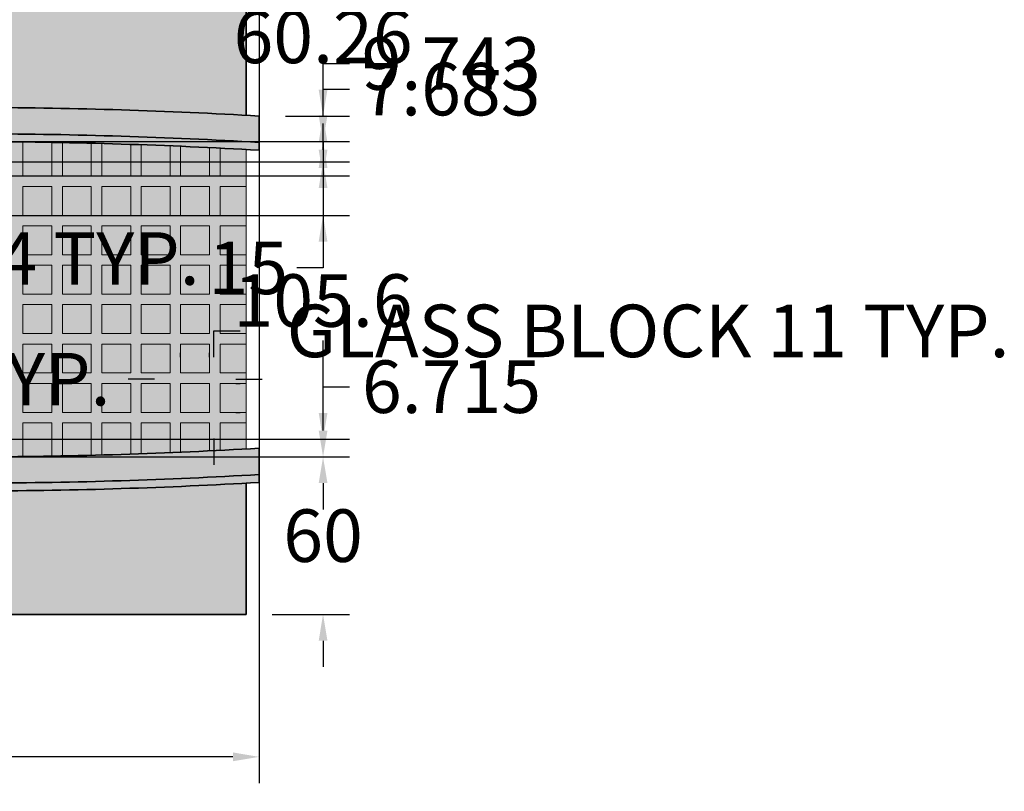
# Model space of a CAD drawing. Units: millimetres. Extents: x 130 to 1021, y 147 to 699.
# Tile 39 of 40: x 646 to 1021, y 147 to 440. Entities that reach past the tile are written whole.
import ezdxf

# ---------------------------------------------------------------- set-up
doc = ezdxf.new("R2010")
doc.units = ezdxf.units.MM
doc.header["$MEASUREMENT"] = 0
for name, color, linetype, lineweight in [('A-ANNO-DIMS', 2, 'Continuous', 18), ('A-ELEV', 7, 'Continuous', 35), ('A-ELEV-PATT', 9, 'Continuous', 13), ('A-GLAZ', 4, 'Continuous', 18)]:
    doc.layers.add(name, color=color, linetype=linetype, lineweight=lineweight)
doc.styles.get("Standard").update_dxf_attribs({"font": 'arial.ttf'})
doc.dimstyles.get("Standard").update_dxf_attribs({"dimtxt": 20, "dimasz": 10, "dimexe": 10, "dimexo": 10, "dimgap": 5, "dimtad": 0, "dimtih": 1, "dimtoh": 1, "dimdec": 0, "dimzin": 0, "dimdsep": 46, "dimtxsty": 'Standard', "dimcen": 5, "dimadec": 0, "dimazin": 0, "dimtfac": 1, "dimtdec": 0, "dimtofl": 0, "dimtmove": 0, "dimatfit": 3, "dimfxl": 1, "dimtolj": 1, "dimtzin": 0, "dimarcsym": 0})

# ---------------------------------------------------------------- blocks, each defined once
blk = doc.blocks.new('GLASS-BLOCK')
for p, q in [((0, 0), (0, 11)), ((0, 11), (11, 11)), ((11, 0), (11, 11)), ((0, 0), (11, 0))]:
    blk.add_line(p, q)
blk = doc.blocks.new('*D5')
at = {"layer": 'A-ANNO-DIMS', "color": 0, "lineweight": -2, "transparency": 16777216}
for p, q in [((720.13, 311.89), (720.13, 321.89)), ((720.13, 321.89), (730.13, 321.89)), ((728.48, 301.89), (730.13, 301.89)), ((728.48, 290.89), (730.13, 290.89)), ((720.13, 280.89), (720.13, 270.89))]:
    blk.add_line(p, q, dxfattribs=at)
at = {"layer": 'A-ANNO-DIMS', "color": 0, "transparency": 16777216}
for points in [[(718.46, 311.89), (721.8, 311.89), (720.13, 301.89)], [(718.46, 280.89), (721.8, 280.89), (720.13, 290.89)]]:
    blk.add_solid(points, dxfattribs=at)
at = {"layer": 'Defpoints', "color": 0, "transparency": 16777216}
for p in [(718.48, 301.89), (720.13, 301.89), (718.48, 290.89)]:
    blk.add_point(p, dxfattribs=at)
at = {"layer": 'A-ANNO-DIMS', "color": 0, "transparency": 16777216, "insert": (885.35, 321.89), "char_height": 20, "attachment_point": 5}
blk.add_mtext('\\A1;GLASS BLOCK 11 TYP.', dxfattribs=at)
blk = doc.blocks.new('*D6')
at = {"layer": 'A-ANNO-DIMS', "color": 0, "lineweight": -2, "transparency": 16777216}
for p, q in [((707.48, 311.89), (707.48, 313.54)), ((718.48, 311.89), (718.48, 313.54)), ((697.48, 303.54), (687.48, 303.54)), ((728.48, 303.54), (738.48, 303.54))]:
    blk.add_line(p, q, dxfattribs=at)
at = {"layer": 'A-ANNO-DIMS', "color": 0, "transparency": 16777216}
for points in [[(697.48, 305.21), (697.48, 301.87), (707.48, 303.54)], [(728.48, 305.21), (728.48, 301.87), (718.48, 303.54)]]:
    blk.add_solid(points, dxfattribs=at)
at = {"layer": 'Defpoints', "color": 0, "transparency": 16777216}
for p in [(707.48, 303.54), (707.48, 301.89), (718.48, 301.89)]:
    blk.add_point(p, dxfattribs=at)
at = {"layer": 'A-ANNO-DIMS', "color": 0, "transparency": 16777216, "insert": (634.74, 303.54), "char_height": 20, "attachment_point": 5}
blk.add_mtext('\\A1;11 TYP.', dxfattribs=at)
blk = doc.blocks.new('*D7')
at = {"layer": 'A-ANNO-DIMS', "color": 0, "lineweight": -2, "transparency": 16777216}
for p, q in [((399.37, 349.45), (413.37, 349.45)), ((423.37, 349.45), (433.37, 349.45)), ((389.37, 344.55), (389.37, 339.45)), ((423.37, 344.55), (423.37, 339.45))]:
    blk.add_line(p, q, dxfattribs=at)
at = {"layer": 'A-ANNO-DIMS', "color": 0, "transparency": 16777216}
for points in [[(399.37, 351.11), (399.37, 347.78), (389.37, 349.45)], [(413.37, 351.11), (413.37, 347.78), (423.37, 349.45)]]:
    blk.add_solid(points, dxfattribs=at)
at = {"layer": 'Defpoints', "color": 0, "transparency": 16777216}
for p in [(389.37, 354.55), (423.37, 354.55), (423.37, 349.45)]:
    blk.add_point(p, dxfattribs=at)
at = {"layer": 'A-ANNO-DIMS', "color": 0, "transparency": 16777216, "insert": (582.04, 349.45), "char_height": 20, "attachment_point": 5}
blk.add_mtext('\\A1;DOOR PANEL 34 TYP.', dxfattribs=at)
blk = doc.blocks.new('*D11')
at = {"layer": 'A-ANNO-DIMS', "color": 0, "lineweight": -2, "transparency": 16777216}
for p, q in [((737.37, 648.7), (737.37, 149.74)), ((299.37, 566.95), (299.37, 149.74)), ((309.37, 159.74), (490.86, 159.74)), ((727.37, 159.74), (545.89, 159.74))]:
    blk.add_line(p, q, dxfattribs=at)
at = {"layer": 'A-ANNO-DIMS', "color": 0, "transparency": 16777216}
for points in [[(309.37, 161.41), (309.37, 158.07), (299.37, 159.74)], [(727.37, 161.41), (727.37, 158.07), (737.37, 159.74)]]:
    blk.add_solid(points, dxfattribs=at)
at = {"layer": 'Defpoints', "color": 0, "transparency": 16777216}
for p in [(737.37, 658.7), (299.37, 576.95), (737.37, 159.74)]:
    blk.add_point(p, dxfattribs=at)
at = {"layer": 'A-ANNO-DIMS', "color": 0, "transparency": 16777216, "insert": (518.37, 159.74), "char_height": 20, "attachment_point": 5}
blk.add_mtext('\\A1;438', dxfattribs=at)
blk = doc.blocks.new('*D49')
at = {"layer": 'A-ANNO-DIMS', "color": 0, "lineweight": -2, "transparency": 16777216}
for p, q in [((761.67, 283.95), (761.67, 293.95)), ((642.82, 273.95), (771.67, 273.95)), ((742.37, 213.95), (771.67, 213.95)), ((761.67, 203.95), (761.67, 193.95))]:
    blk.add_line(p, q, dxfattribs=at)
at = {"layer": 'A-ANNO-DIMS', "color": 0, "transparency": 16777216}
for points in [[(760.01, 283.95), (763.34, 283.95), (761.67, 273.95)], [(760.01, 203.95), (763.34, 203.95), (761.67, 213.95)]]:
    blk.add_solid(points, dxfattribs=at)
at = {"layer": 'Defpoints', "color": 0, "transparency": 16777216}
for p in [(632.82, 273.95), (761.67, 273.95), (732.37, 213.95)]:
    blk.add_point(p, dxfattribs=at)
at = {"layer": 'A-ANNO-DIMS', "color": 0, "transparency": 16777216, "insert": (761.67, 243.95), "char_height": 20, "attachment_point": 5}
blk.add_mtext('\\A1;60', dxfattribs=at)
blk = doc.blocks.new('*D50')
at = {"layer": 'A-ANNO-DIMS', "color": 0, "lineweight": -2, "transparency": 16777216}
for p, q in [((761.67, 290.66), (761.67, 300.66)), ((761.67, 300.66), (771.67, 300.66)), ((554.64, 280.66), (771.67, 280.66)), ((642.82, 273.95), (771.67, 273.95)), ((761.67, 263.95), (761.67, 253.95))]:
    blk.add_line(p, q, dxfattribs=at)
at = {"layer": 'A-ANNO-DIMS', "color": 0, "transparency": 16777216}
for points in [[(760.01, 290.66), (763.34, 290.66), (761.67, 280.66)], [(760.01, 263.95), (763.34, 263.95), (761.67, 273.95)]]:
    blk.add_solid(points, dxfattribs=at)
at = {"layer": 'Defpoints', "color": 0, "transparency": 16777216}
for p in [(544.64, 280.66), (761.67, 280.66), (632.82, 273.95)]:
    blk.add_point(p, dxfattribs=at)
at = {"layer": 'A-ANNO-DIMS', "color": 0, "transparency": 16777216, "insert": (810.55, 300.66), "char_height": 20, "attachment_point": 5}
blk.add_mtext('\\A1;6.715', dxfattribs=at)
blk = doc.blocks.new('*D51')
at = {"layer": 'A-ANNO-DIMS', "color": 0, "lineweight": -2, "transparency": 16777216}
for p, q in [((554.64, 386.26), (771.67, 386.26)), ((761.67, 376.26), (761.67, 348.67)), ((761.67, 290.66), (761.67, 318.25)), ((554.64, 280.66), (771.67, 280.66))]:
    blk.add_line(p, q, dxfattribs=at)
at = {"layer": 'A-ANNO-DIMS', "color": 0, "transparency": 16777216}
for points in [[(760.01, 376.26), (763.34, 376.26), (761.67, 386.26)], [(760.01, 290.66), (763.34, 290.66), (761.67, 280.66)]]:
    blk.add_solid(points, dxfattribs=at)
at = {"layer": 'Defpoints', "color": 0, "transparency": 16777216}
for p in [(544.64, 386.26), (761.67, 386.26), (544.64, 280.66)]:
    blk.add_point(p, dxfattribs=at)
at = {"layer": 'A-ANNO-DIMS', "color": 0, "transparency": 16777216, "insert": (761.67, 333.46), "char_height": 20, "attachment_point": 5}
blk.add_mtext('\\A1;105.6', dxfattribs=at)
blk = doc.blocks.new('*D52')
at = {"layer": 'A-ANNO-DIMS', "color": 0, "lineweight": -2, "transparency": 16777216}
for p, q in [((761.67, 403.95), (761.67, 413.95)), ((761.67, 413.95), (771.67, 413.95)), ((642.82, 393.95), (771.67, 393.95)), ((554.64, 386.26), (771.67, 386.26)), ((761.67, 376.26), (761.67, 366.26))]:
    blk.add_line(p, q, dxfattribs=at)
at = {"layer": 'A-ANNO-DIMS', "color": 0, "transparency": 16777216}
for points in [[(760.01, 403.95), (763.34, 403.95), (761.67, 393.95)], [(760.01, 376.26), (763.34, 376.26), (761.67, 386.26)]]:
    blk.add_solid(points, dxfattribs=at)
at = {"layer": 'Defpoints', "color": 0, "transparency": 16777216}
for p in [(632.82, 393.95), (761.67, 393.95), (544.64, 386.26)]:
    blk.add_point(p, dxfattribs=at)
at = {"layer": 'A-ANNO-DIMS', "color": 0, "transparency": 16777216, "insert": (810.34, 413.95), "char_height": 20, "attachment_point": 5}
blk.add_mtext('\\A1;7.683', dxfattribs=at)
blk = doc.blocks.new('*D53')
at = {"layer": 'A-ANNO-DIMS', "color": 0, "lineweight": -2, "transparency": 16777216}
for p, q in [((761.67, 413.69), (761.67, 423.69)), ((761.67, 423.69), (771.67, 423.69)), ((747.37, 403.69), (771.67, 403.69)), ((642.82, 393.95), (771.67, 393.95)), ((761.67, 383.95), (761.67, 373.95))]:
    blk.add_line(p, q, dxfattribs=at)
at = {"layer": 'A-ANNO-DIMS', "color": 0, "transparency": 16777216}
for points in [[(760.01, 413.69), (763.34, 413.69), (761.67, 403.69)], [(760.01, 383.95), (763.34, 383.95), (761.67, 393.95)]]:
    blk.add_solid(points, dxfattribs=at)
at = {"layer": 'Defpoints', "color": 0, "transparency": 16777216}
for p in [(737.37, 403.69), (761.67, 403.69), (632.82, 393.95)]:
    blk.add_point(p, dxfattribs=at)
at = {"layer": 'A-ANNO-DIMS', "color": 0, "transparency": 16777216, "insert": (810.42, 423.69), "char_height": 20, "attachment_point": 5}
blk.add_mtext('\\A1;9.743', dxfattribs=at)
blk = doc.blocks.new('*D54')
at = {"layer": 'A-ANNO-DIMS', "color": 0, "lineweight": -2, "transparency": 16777216}
for p, q in [((761.67, 473.95), (761.67, 483.95)), ((497.37, 463.95), (771.67, 463.95)), ((747.37, 403.69), (771.67, 403.69)), ((761.67, 393.69), (761.67, 383.69))]:
    blk.add_line(p, q, dxfattribs=at)
at = {"layer": 'A-ANNO-DIMS', "color": 0, "transparency": 16777216}
for points in [[(760.01, 473.95), (763.34, 473.95), (761.67, 463.95)], [(760.01, 393.69), (763.34, 393.69), (761.67, 403.69)]]:
    blk.add_solid(points, dxfattribs=at)
at = {"layer": 'Defpoints', "color": 0, "transparency": 16777216}
for p in [(487.37, 463.95), (761.67, 463.95), (737.37, 403.69)]:
    blk.add_point(p, dxfattribs=at)
at = {"layer": 'A-ANNO-DIMS', "color": 0, "transparency": 16777216, "insert": (761.67, 433.82), "char_height": 20, "attachment_point": 5}
blk.add_mtext('\\A1;60.26', dxfattribs=at)
blk = doc.blocks.new('*D61')
at = {"layer": 'A-ANNO-DIMS', "color": 0, "lineweight": -2, "transparency": 16777216}
for p, q in [((761.67, 390.89), (761.67, 400.89)), ((642.82, 380.89), (771.67, 380.89)), ((642.82, 365.89), (771.67, 365.89)), ((761.67, 355.89), (761.67, 345.89)), ((761.67, 345.89), (751.67, 345.89))]:
    blk.add_line(p, q, dxfattribs=at)
at = {"layer": 'A-ANNO-DIMS', "color": 0, "transparency": 16777216}
for points in [[(760.01, 390.89), (763.34, 390.89), (761.67, 380.89)], [(760.01, 355.89), (763.34, 355.89), (761.67, 365.89)]]:
    blk.add_solid(points, dxfattribs=at)
at = {"layer": 'Defpoints', "color": 0, "transparency": 16777216}
for p in [(632.82, 380.89), (632.82, 365.89), (761.67, 365.89)]:
    blk.add_point(p, dxfattribs=at)
at = {"layer": 'A-ANNO-DIMS', "color": 0, "transparency": 16777216, "insert": (733.22, 345.89), "char_height": 20, "attachment_point": 5}
blk.add_mtext('\\A1;15', dxfattribs=at)

msp = doc.modelspace()

# ---------------------------------------------------------------- hatches: boundary and pattern name
at = {"layer": 'A-ELEV-PATT'}
h = msp.add_hatch(color=256, dxfattribs=at)
h.dxf.hatch_style = 1
h.paths.add_polyline_path([(737.3738, 658.6988, 0.01359606), (632.4019, 661.9473), (607.3738, 661.9473), (487.3738, 661.9473), (487.3738, 649.9473), (607.3738, 649.9473), (632.3794, 649.9473, -0.01368411), (737.3738, 646.6784)])
h.paths.add_polyline_path([(732.3738, 643.9599, 0.01305286), (632.3738, 646.9473), (607.3738, 646.9473), (487.3738, 646.9473), (487.3738, 596.9473), (632.3738, 596.9473, -0.01305286), (732.3738, 593.9599)])
h.paths.add_polyline_path([(737.3738, 593.6732, 0.01370629), (632.3738, 596.9473), (487.3738, 596.9473), (487.3738, 586.9473), (632.355, 586.9473, -0.01378075), (737.3738, 583.6559)])
h.paths.add_polyline_path([(447.3738, 646.9473), (307.3738, 646.9473), (302.3738, 646.9473), (302.3738, 634.9473), (447.3738, 634.9473)])
h.paths.add_polyline_path([(447.3738, 631.9473), (307.3738, 631.9473), (307.3738, 586.9473), (447.3738, 586.9473)])
h.paths.add_polyline_path([(447.3738, 586.9473), (307.3738, 586.9473), (302.3738, 586.9473), (302.3738, 576.9473), (447.3738, 576.9473)])
h.paths.add_polyline_path([(447.3738, 573.9473), (367.3738, 573.9473), (367.3738, 539.9473), (447.3738, 539.9473)])
h.paths.add_polyline_path([(447.3738, 537.9473), (367.3738, 537.9473), (367.3738, 507.9473), (400.392, 507.4253, -0.00172798), (401.3281, 507.6451, -0.52200255), (425.6117, 511.0391, -0.03918489), (447.3738, 510.4359), (447.3738, 510.7883)])
h.paths.add_polyline_path([(394.7238, 505.9473), (367.3738, 505.9473), (367.3738, 476.9473, -0.0146512), (375.8501, 480.2159), (376.1506, 499.2266, -0.03554194)])
h.paths.add_polyline_path([(632.3738, 583.9473), (552.3738, 583.9473), (552.3738, 550.9473), (632.3738, 550.9473)])
h.paths.add_polyline_path([(632.3738, 548.9473), (552.3738, 548.9473), (552.3738, 515.9473), (632.3738, 515.9473)])
h.paths.add_polyline_path([(632.3738, 513.9473), (552.3738, 513.9473), (552.3738, 476.9473), (632.3738, 476.9473)])
h.paths.add_polyline_path([(737.3738, 473.6903, 0.01363261), (632.3926, 476.9473), (552.3738, 476.9473), (487.3738, 476.9473), (487.3738, 466.9473), (632.3738, 466.9473, -0.01370629), (737.3738, 463.6732)])
h.paths.add_polyline_path([(732.3738, 460.9552, 0.01307409), (632.3681, 463.9473), (487.3738, 463.9473), (487.3738, 407.735, -0.00322862), (489.3544, 406.9473), (632.3926, 406.9473, -0.01298259), (732.3738, 403.9755)])
h.paths.add_polyline_path([(487.3738, 463.9473, 0.20132998), (367.3738, 463.9473), (367.3738, 407.735, -0.18820307), (487.3738, 407.735)])
h.paths.add_polyline_path([(367.3738, 476.9473), (367.3738, 466.9473, -0.20133085), (487.3738, 466.9473), (487.3738, 476.9473, 0.20132998)])
h.paths.add_polyline_path([(367.3738, 463.9473), (307.3738, 463.9473), (307.3738, 401.9473), (357.9413, 401.9473), (367.3738, 407.735)])
h.paths.add_polyline_path([(367.3738, 476.9473), (302.3738, 476.9473), (302.3738, 466.9473), (367.3738, 466.9473)])
h.paths.add_polyline_path([(632.8184, 366.9453), (552.3738, 366.9453), (552.3738, 393.9473), (632.8184, 393.9473)])
h.paths.add_polyline_path([(632.8184, 357.2114), (632.8184, 363.9453), (552.3738, 363.9453), (552.3738, 357.2114), (552.3738, 336.9453), (632.8184, 336.9453)])
h.paths.add_polyline_path([(632.8184, 333.9453), (552.3738, 333.9453), (552.3738, 306.9453), (632.8184, 306.9453)])
h.paths.add_polyline_path([(632.8184, 303.9453), (552.3738, 303.9453), (552.3738, 273.9473), (632.355, 273.9473, 0.00006077), (632.8184, 273.9491)])
h.paths.add_polyline_path([(737.3738, 403.6903, 0.01363261), (632.3926, 406.9473), (489.3544, 406.9473, 0.19154808), (367.3738, 407.735), (367.3738, 396.9473, -0.20133085), (487.3738, 396.9473), (632.3738, 396.9473, -0.01370629), (737.3738, 393.6732)])
h.paths.add_polyline_path([(357.9413, 401.9473), (307.3738, 401.9473), (307.3738, 391.9473), (357.9413, 391.9473)])
h.paths.add_polyline_path([(357.9413, 357.2114), (357.9413, 388.9473), (307.3738, 388.9473), (307.3738, 357.2114), (307.3738, 273.9473), (357.9413, 273.9473)])
h.paths.add_polyline_path([(732.3738, 263.93, -0.0130317), (632.3794, 260.9473), (466.7667, 260.9473), (466.7667, 240.9473), (469.8406, 236.978), (469.8406, 221.978), (472.9145, 218.0087), (472.9145, 213.9473), (607.3738, 213.9473), (732.3738, 213.9473)])
h.paths.add_polyline_path([(732.3738, 290.889), (722.479, 290.889), (722.479, 301.889), (732.3738, 301.889), (732.3738, 305.889), (722.479, 305.889), (722.479, 316.889), (732.3738, 316.889), (732.3738, 320.889), (722.479, 320.889), (722.479, 331.889), (732.3738, 331.889), (732.3738, 335.889), (722.479, 335.889), (722.479, 346.889), (732.3738, 346.889), (732.3738, 350.889), (722.479, 350.889), (722.479, 361.889), (732.3738, 361.889), (732.3738, 365.889), (722.479, 365.889), (722.479, 376.889), (732.3738, 376.889), (732.3738, 380.889), (722.479, 380.889), (722.479, 391.4848, 0.00052326), (718.479, 391.6843), (718.479, 380.889), (707.479, 380.889), (707.479, 392.1896, 0.00052307), (703.479, 392.3576), (703.479, 380.889), (692.479, 380.889), (692.479, 392.7765, 0.00052292), (688.479, 392.9131), (688.479, 380.889), (677.479, 380.889), (677.479, 393.2456, 0.00052279), (673.479, 393.3508), (673.479, 380.889), (662.479, 380.889), (662.479, 393.597, 0.0005227), (658.479, 393.6709), (658.479, 380.889), (647.479, 380.889), (647.479, 393.8308, 0.00052264), (643.479, 393.8732), (643.479, 380.889), (632.8184, 380.889), (632.8184, 376.889), (643.479, 376.889), (643.479, 365.889), (632.8184, 365.889), (632.8184, 361.889), (643.479, 361.889), (643.479, 350.889), (632.8184, 350.889), (632.8184, 346.889), (643.479, 346.889), (643.479, 335.889), (632.8184, 335.889), (632.8184, 331.889), (643.479, 331.889), (643.479, 320.889), (632.8184, 320.889), (632.8184, 316.889), (643.479, 316.889), (643.479, 305.889), (632.8184, 305.889), (632.8184, 301.889), (643.479, 301.889), (643.479, 290.889), (632.8184, 290.889), (632.8184, 286.889), (643.479, 286.889), (643.479, 274.0217, 0.00052456), (647.479, 274.0643), (647.479, 286.889), (658.479, 286.889), (658.479, 274.2248, 0.00052462), (662.479, 274.2989), (662.479, 286.889), (673.479, 286.889), (673.479, 274.546, 0.00052471), (677.479, 274.6516), (677.479, 286.889), (688.479, 286.889), (688.479, 274.9853, 0.00052484), (692.479, 275.1224), (692.479, 286.889), (703.479, 286.889), (703.479, 275.5429, 0.000525), (707.479, 275.7115), (707.479, 286.889), (718.479, 286.889), (718.479, 276.2187, 0.00052519), (722.479, 276.4189), (722.479, 286.889), (732.3738, 286.889)])
h.paths.add_polyline_path([(718.479, 290.889), (707.479, 290.889), (707.479, 301.889), (718.479, 301.889)], flags=16)
h.paths.add_polyline_path([(703.479, 290.889), (692.479, 290.889), (692.479, 301.889), (703.479, 301.889)], flags=16)
h.paths.add_polyline_path([(718.479, 305.889), (707.479, 305.889), (707.479, 316.889), (718.479, 316.889)], flags=16)
h.paths.add_polyline_path([(703.479, 305.889), (692.479, 305.889), (692.479, 316.889), (703.479, 316.889)], flags=16)
h.paths.add_polyline_path([(688.479, 290.889), (677.479, 290.889), (677.479, 301.889), (688.479, 301.889)], flags=16)
h.paths.add_polyline_path([(718.479, 320.889), (707.479, 320.889), (707.479, 331.889), (718.479, 331.889)], flags=16)
h.paths.add_polyline_path([(688.479, 305.889), (677.479, 305.889), (677.479, 316.889), (688.479, 316.889)], flags=16)
h.paths.add_polyline_path([(703.479, 320.889), (692.479, 320.889), (692.479, 331.889), (703.479, 331.889)], flags=16)
h.paths.add_polyline_path([(688.479, 320.889), (677.479, 320.889), (677.479, 331.889), (688.479, 331.889)], flags=16)
h.paths.add_polyline_path([(673.479, 290.889), (662.479, 290.889), (662.479, 301.889), (673.479, 301.889)], flags=16)
h.paths.add_polyline_path([(718.479, 335.889), (707.479, 335.889), (707.479, 346.889), (718.479, 346.889)], flags=16)
h.paths.add_polyline_path([(673.479, 305.889), (662.479, 305.889), (662.479, 316.889), (673.479, 316.889)], flags=16)
h.paths.add_polyline_path([(703.479, 335.889), (692.479, 335.889), (692.479, 346.889), (703.479, 346.889)], flags=16)
h.paths.add_polyline_path([(673.479, 320.889), (662.479, 320.889), (662.479, 331.889), (673.479, 331.889)], flags=16)
h.paths.add_polyline_path([(688.479, 335.889), (677.479, 335.889), (677.479, 346.889), (688.479, 346.889)], flags=16)
h.paths.add_polyline_path([(658.479, 290.889), (647.479, 290.889), (647.479, 301.889), (658.479, 301.889)], flags=16)
h.paths.add_polyline_path([(718.479, 350.889), (707.479, 350.889), (707.479, 361.889), (718.479, 361.889)], flags=16)
h.paths.add_polyline_path([(658.479, 305.889), (647.479, 305.889), (647.479, 316.889), (658.479, 316.889)], flags=16)
h.paths.add_polyline_path([(703.479, 350.889), (692.479, 350.889), (692.479, 361.889), (703.479, 361.889)], flags=16)
h.paths.add_polyline_path([(673.479, 335.889), (662.479, 335.889), (662.479, 346.889), (673.479, 346.889)], flags=16)
h.paths.add_polyline_path([(658.479, 320.889), (647.479, 320.889), (647.479, 331.889), (658.479, 331.889)], flags=16)
h.paths.add_polyline_path([(688.479, 350.889), (677.479, 350.889), (677.479, 361.889), (688.479, 361.889)], flags=16)
h.paths.add_polyline_path([(718.479, 365.889), (707.479, 365.889), (707.479, 376.889), (718.479, 376.889)], flags=16)
h.paths.add_polyline_path([(658.479, 335.889), (647.479, 335.889), (647.479, 346.889), (658.479, 346.889)], flags=16)
h.paths.add_polyline_path([(673.479, 350.889), (662.479, 350.889), (662.479, 361.889), (673.479, 361.889)], flags=16)
h.paths.add_polyline_path([(703.479, 365.889), (692.479, 365.889), (692.479, 376.889), (703.479, 376.889)], flags=16)
h.paths.add_polyline_path([(688.479, 365.889), (677.479, 365.889), (677.479, 376.889), (688.479, 376.889)], flags=16)
h.paths.add_polyline_path([(658.479, 350.889), (647.479, 350.889), (647.479, 361.889), (658.479, 361.889)], flags=16)
h.paths.add_polyline_path([(673.479, 365.889), (662.479, 365.889), (662.479, 376.889), (673.479, 376.889)], flags=16)
h.paths.add_polyline_path([(658.479, 365.889), (647.479, 365.889), (647.479, 376.889), (658.479, 376.889)], flags=16)
h.paths.add_polyline_path([(732.3738, 503.9786), (722.3392, 503.9786), (722.3392, 514.9786), (732.3738, 514.9786), (732.3738, 518.9786), (722.3392, 518.9786), (722.3392, 529.9786), (732.3738, 529.9786), (732.3738, 533.9786), (722.3392, 533.9786), (722.3392, 544.9786), (732.3738, 544.9786), (732.3738, 546.9473), (732.3738, 548.9786), (722.3392, 548.9786), (722.3392, 559.9786), (732.3738, 559.9786), (732.3738, 563.9786), (722.3392, 563.9786), (722.3392, 574.9786), (732.3738, 574.9786), (732.3738, 578.9786), (722.3392, 578.9786), (722.3392, 581.4789, 0.00052601), (718.3392, 581.6791), (718.3392, 578.9786), (707.3392, 578.9786), (707.3392, 582.1863, 0.00052582), (703.3392, 582.355), (703.3392, 578.9786), (692.3392, 578.9786), (692.3392, 582.7752, 0.00052566), (688.3392, 582.9123), (688.3392, 578.9786), (677.3392, 578.9786), (677.3392, 583.2457, 0.00052554), (673.3392, 583.3512), (673.3392, 578.9786), (662.3392, 578.9786), (662.3392, 583.5978, 0.00052545), (658.3392, 583.6718), (658.3392, 578.9786), (647.3392, 578.9786), (647.3392, 583.8317, 0.00052539), (643.3392, 583.8741), (643.3392, 578.9786), (632.3738, 578.9786), (632.3738, 574.9786), (643.3392, 574.9786), (643.3392, 563.9786), (632.3738, 563.9786), (632.3738, 559.9786), (643.3392, 559.9786), (643.3392, 548.9786), (632.3738, 548.9786), (632.3738, 544.9786), (643.3392, 544.9786), (643.3392, 533.9786), (632.3738, 533.9786), (632.3738, 529.9786), (643.3392, 529.9786), (643.3392, 518.9786), (632.3738, 518.9786), (632.3738, 515.9473), (632.3738, 514.9786), (643.3392, 514.9786), (643.3392, 503.9786), (632.3738, 503.9786), (632.3738, 499.9786), (643.3392, 499.9786), (643.3392, 488.9786), (632.3738, 488.9786), (632.3738, 484.9786), (643.3392, 484.9786), (643.3392, 476.8751, -0.00051911), (647.3392, 476.8332), (647.3392, 484.9786), (658.3392, 484.9786), (658.3392, 476.6752, -0.00051917), (662.3392, 476.6022), (662.3392, 484.9786), (673.3392, 484.9786), (673.3392, 476.3585, -0.00051926), (677.3392, 476.2543), (677.3392, 484.9786), (688.3392, 484.9786), (688.3392, 475.9248, -0.00051938), (692.3392, 475.7894), (692.3392, 484.9786), (703.3392, 484.9786), (703.3392, 475.3741, -0.00051953), (707.3392, 475.2075), (707.3392, 484.9786), (718.3392, 484.9786), (718.3392, 474.7064, -0.00051972), (722.3392, 474.5086), (722.3392, 484.9786), (732.3738, 484.9786), (732.3738, 488.9786), (722.3392, 488.9786), (722.3392, 499.9786), (732.3738, 499.9786)])
h.paths.add_polyline_path([(718.3392, 503.9786), (707.3392, 503.9786), (707.3392, 514.9786), (718.3392, 514.9786)], flags=16)
h.paths.add_polyline_path([(718.3392, 499.9786), (718.3392, 488.9786), (707.3392, 488.9786), (707.3392, 499.9786)], flags=16)
h.paths.add_polyline_path([(718.3392, 518.9786), (707.3392, 518.9786), (707.3392, 529.9786), (718.3392, 529.9786)], flags=16)
h.paths.add_polyline_path([(703.3392, 503.9786), (692.3392, 503.9786), (692.3392, 514.9786), (703.3392, 514.9786)], flags=16)
h.paths.add_polyline_path([(703.3392, 499.9786), (703.3392, 488.9786), (692.3392, 488.9786), (692.3392, 499.9786)], flags=16)
h.paths.add_polyline_path([(703.3392, 518.9786), (692.3392, 518.9786), (692.3392, 529.9786), (703.3392, 529.9786)], flags=16)
h.paths.add_polyline_path([(718.3392, 533.9786), (707.3392, 533.9786), (707.3392, 544.9786), (718.3392, 544.9786)], flags=16)
h.paths.add_polyline_path([(688.3392, 503.9786), (677.3392, 503.9786), (677.3392, 514.9786), (688.3392, 514.9786)], flags=16)
h.paths.add_polyline_path([(688.3392, 499.9786), (688.3392, 488.9786), (677.3392, 488.9786), (677.3392, 499.9786)], flags=16)
h.paths.add_polyline_path([(703.3392, 533.9786), (692.3392, 533.9786), (692.3392, 544.9786), (703.3392, 544.9786)], flags=16)
h.paths.add_polyline_path([(688.3392, 518.9786), (677.3392, 518.9786), (677.3392, 529.9786), (688.3392, 529.9786)], flags=16)
h.paths.add_polyline_path([(688.3392, 533.9786), (677.3392, 533.9786), (677.3392, 544.9786), (688.3392, 544.9786)], flags=16)
h.paths.add_polyline_path([(718.3392, 548.9786), (707.3392, 548.9786), (707.3392, 559.9786), (718.3392, 559.9786)], flags=16)
h.paths.add_polyline_path([(673.3392, 503.9786), (662.3392, 503.9786), (662.3392, 514.9786), (673.3392, 514.9786)], flags=16)
h.paths.add_polyline_path([(673.3392, 499.9786), (673.3392, 488.9786), (662.3392, 488.9786), (662.3392, 499.9786)], flags=16)
h.paths.add_polyline_path([(703.3392, 548.9786), (692.3392, 548.9786), (692.3392, 559.9786), (703.3392, 559.9786)], flags=16)
h.paths.add_polyline_path([(673.3392, 518.9786), (662.3392, 518.9786), (662.3392, 529.9786), (673.3392, 529.9786)], flags=16)
h.paths.add_polyline_path([(688.3392, 548.9786), (677.3392, 548.9786), (677.3392, 559.9786), (688.3392, 559.9786)], flags=16)
h.paths.add_polyline_path([(673.3392, 533.9786), (662.3392, 533.9786), (662.3392, 544.9786), (673.3392, 544.9786)], flags=16)
h.paths.add_polyline_path([(718.3392, 563.9786), (707.3392, 563.9786), (707.3392, 574.9786), (718.3392, 574.9786)], flags=16)
h.paths.add_polyline_path([(658.3392, 503.9786), (647.3392, 503.9786), (647.3392, 514.9786), (658.3392, 514.9786)], flags=16)
h.paths.add_polyline_path([(658.3392, 499.9786), (658.3392, 488.9786), (647.3392, 488.9786), (647.3392, 499.9786)], flags=16)
h.paths.add_polyline_path([(703.3392, 563.9786), (692.3392, 563.9786), (692.3392, 574.9786), (703.3392, 574.9786)], flags=16)
h.paths.add_polyline_path([(658.3392, 518.9786), (647.3392, 518.9786), (647.3392, 529.9786), (658.3392, 529.9786)], flags=16)
h.paths.add_polyline_path([(673.3392, 548.9786), (662.3392, 548.9786), (662.3392, 559.9786), (673.3392, 559.9786)], flags=16)
h.paths.add_polyline_path([(688.3392, 563.9786), (677.3392, 563.9786), (677.3392, 574.9786), (688.3392, 574.9786)], flags=16)
h.paths.add_polyline_path([(658.3392, 533.9786), (647.3392, 533.9786), (647.3392, 544.9786), (658.3392, 544.9786)], flags=16)
h.paths.add_polyline_path([(673.3392, 563.9786), (662.3392, 563.9786), (662.3392, 574.9786), (673.3392, 574.9786)], flags=16)
h.paths.add_polyline_path([(658.3392, 548.9786), (647.3392, 548.9786), (647.3392, 559.9786), (658.3392, 559.9786)], flags=16)
h.paths.add_polyline_path([(658.3392, 563.9786), (647.3392, 563.9786), (647.3392, 574.9786), (658.3392, 574.9786)], flags=16)
h = msp.add_hatch(color=256, dxfattribs=at)
h.dxf.hatch_style = 1
h.paths.add_polyline_path([(447.3738, 576.9473), (302.3738, 576.9473), (302.3738, 573.9473), (447.3738, 573.9473)])
h.paths.add_polyline_path([(487.3738, 583.9473), (487.3738, 586.9473), (447.3738, 576.9473), (447.3738, 573.9473)])
h.paths.add_polyline_path([(632.355, 586.9473), (487.3738, 586.9473), (487.3738, 583.9473), (632.3738, 583.9473), (632.3738, 583.9472, -0.01380003), (737.3738, 580.6507), (737.3738, 583.6559, 0.01378075)])
h.paths.add_polyline_path([(367.3738, 466.9473), (302.3738, 466.9473), (302.3738, 463.9473), (367.3738, 463.9473)])
h.paths.add_polyline_path([(487.3738, 463.9473), (487.3738, 466.9473, 0.20133085), (367.3738, 466.9473), (367.3738, 463.9473, -0.20132998)])
h.paths.add_polyline_path([(632.3738, 466.9473), (487.3738, 466.9473), (487.3738, 463.9473), (632.3681, 463.9473, -0.01372855), (737.3738, 460.6681), (737.3738, 463.6732, 0.01370629)])
h.paths.add_polyline_path([(632.3738, 396.9473), (487.3738, 396.9473, 0.20133085), (367.3738, 396.9473), (367.3738, 393.9473, -0.20237172), (486.7667, 393.9473), (632.3681, 393.9473, -0.01372855), (737.3738, 390.6681), (737.3738, 393.6732, 0.01370629)])
h.paths.add_polyline_path([(357.9413, 391.9473), (307.3738, 391.9473), (307.3738, 388.9473), (357.9413, 388.9473)])
h.paths.add_polyline_path([(367.3738, 393.9473), (367.3738, 396.9473), (357.9413, 391.924), (357.9413, 388.9473), (358.058, 388.9473)])
h.paths.add_polyline_path([(737.3738, 264.2162), (737.3738, 267.2214, -0.01370629), (632.3738, 263.9473), (463.7667, 263.9473), (466.7667, 260.9473), (632.3794, 260.9473, 0.01368411)])
h.paths.add_polyline_path([(463.7667, 263.9473), (447.3738, 263.9473), (450.3738, 260.9473), (466.7667, 260.9473)])
h.paths.add_polyline_path([(447.3738, 263.9473), (432.3738, 263.9473), (432.3738, 260.9473), (450.3738, 260.9473)])
h.paths.add_polyline_path([(382.3738, 263.9473), (357.9413, 263.9473), (357.9413, 260.9473), (382.3738, 260.9473)])
h.paths.add_polyline_path([(357.9413, 263.9473), (307.3738, 263.9473), (307.3738, 260.9473), (357.9413, 260.9473)])
h = msp.add_hatch(color=256, dxfattribs=at)
h.set_gradient(color1=(0, 153, 204), color2=(102, 204, 127))
h.paths.add_polyline_path([(643.479, 286.889), (632.8184, 286.889), (632.8184, 273.9491, 0.00139799), (643.479, 274.0217)])
h.paths.add_polyline_path([(647.479, 274.0643, 0.00144261), (658.479, 274.2248), (658.479, 286.889), (647.479, 286.889)])
h.paths.add_polyline_path([(662.479, 274.2989, 0.00144282), (673.479, 274.546), (673.479, 286.889), (662.479, 286.889)])
h.paths.add_polyline_path([(677.479, 274.6516, 0.00144312), (688.479, 274.9853), (688.479, 286.889), (677.479, 286.889)])
h.paths.add_polyline_path([(703.479, 275.5429), (703.479, 286.889), (692.479, 286.889), (692.479, 275.1224, 0.00144351)])
h.paths.add_polyline_path([(707.479, 275.7115, 0.00144399), (718.479, 276.2187), (718.479, 286.889), (707.479, 286.889)])
h.paths.add_polyline_path([(722.479, 276.4189, 0.0012994), (732.3738, 276.9505), (732.3738, 286.889), (722.479, 286.889)])
h.paths.add_polyline_path([(722.479, 290.889), (732.3738, 290.889), (732.3738, 301.889), (722.479, 301.889)])
h.paths.add_polyline_path([(718.479, 301.889), (707.479, 301.889), (707.479, 290.889), (718.479, 290.889)])
h.paths.add_polyline_path([(703.479, 301.889), (692.479, 301.889), (692.479, 290.889), (703.479, 290.889)])
h.paths.add_polyline_path([(677.479, 290.889), (688.479, 290.889), (688.479, 301.889), (677.479, 301.889)])
h.paths.add_polyline_path([(673.479, 301.889), (662.479, 301.889), (662.479, 290.889), (673.479, 290.889)])
h.paths.add_polyline_path([(658.479, 301.889), (647.479, 301.889), (647.479, 290.889), (658.479, 290.889)])
h.paths.add_polyline_path([(643.479, 301.889), (632.8184, 301.889), (632.8184, 290.889), (643.479, 290.889)])
h.paths.add_polyline_path([(643.479, 316.889), (632.8184, 316.889), (632.8184, 305.889), (643.479, 305.889)])
h.paths.add_polyline_path([(647.479, 305.889), (658.479, 305.889), (658.479, 316.889), (647.479, 316.889)])
h.paths.add_polyline_path([(662.479, 305.889), (673.479, 305.889), (673.479, 316.889), (662.479, 316.889)])
h.paths.add_polyline_path([(688.479, 316.889), (677.479, 316.889), (677.479, 305.889), (688.479, 305.889)])
h.paths.add_polyline_path([(692.479, 305.889), (703.479, 305.889), (703.479, 316.889), (692.479, 316.889)])
h.paths.add_polyline_path([(707.479, 305.889), (718.479, 305.889), (718.479, 316.889), (707.479, 316.889)])
h.paths.add_polyline_path([(722.479, 305.889), (732.3738, 305.889), (732.3738, 316.889), (722.479, 316.889)])
h.paths.add_polyline_path([(732.3738, 331.889), (722.479, 331.889), (722.479, 320.889), (732.3738, 320.889)])
h.paths.add_polyline_path([(718.479, 331.889), (707.479, 331.889), (707.479, 320.889), (718.479, 320.889)])
h.paths.add_polyline_path([(703.479, 331.889), (692.479, 331.889), (692.479, 320.889), (703.479, 320.889)])
h.paths.add_polyline_path([(688.479, 331.889), (677.479, 331.889), (677.479, 320.889), (688.479, 320.889)])
h.paths.add_polyline_path([(673.479, 331.889), (662.479, 331.889), (662.479, 320.889), (673.479, 320.889)])
h.paths.add_polyline_path([(647.479, 320.889), (658.479, 320.889), (658.479, 331.889), (647.479, 331.889)])
h.paths.add_polyline_path([(643.479, 320.889), (643.479, 331.889), (632.8184, 331.889), (632.8184, 320.889)])
h.paths.add_polyline_path([(632.8184, 335.889), (643.479, 335.889), (643.479, 346.889), (632.8184, 346.889)])
h.paths.add_polyline_path([(647.479, 335.889), (658.479, 335.889), (658.479, 346.889), (647.479, 346.889)])
h.paths.add_polyline_path([(673.479, 346.889), (662.479, 346.889), (662.479, 335.889), (673.479, 335.889)])
h.paths.add_polyline_path([(677.479, 335.889), (688.479, 335.889), (688.479, 346.889), (677.479, 346.889)])
h.paths.add_polyline_path([(703.479, 346.889), (692.479, 346.889), (692.479, 335.889), (703.479, 335.889)])
h.paths.add_polyline_path([(707.479, 335.889), (718.479, 335.889), (718.479, 346.889), (707.479, 346.889)])
h.paths.add_polyline_path([(722.479, 335.889), (732.3738, 335.889), (732.3738, 346.889), (722.479, 346.889)])
h.paths.add_polyline_path([(722.479, 361.889), (722.479, 350.889), (732.3738, 350.889), (732.3738, 357.2114), (732.3738, 361.889)])
h.paths.add_polyline_path([(707.479, 350.889), (718.479, 350.889), (718.479, 361.889), (707.479, 361.889)])
h.paths.add_polyline_path([(703.479, 361.889), (692.479, 361.889), (692.479, 350.889), (703.479, 350.889)])
h.paths.add_polyline_path([(688.479, 361.889), (677.479, 361.889), (677.479, 350.889), (688.479, 350.889)])
h.paths.add_polyline_path([(662.479, 350.889), (673.479, 350.889), (673.479, 361.889), (662.479, 361.889)])
h.paths.add_polyline_path([(658.479, 350.889), (658.479, 361.889), (647.479, 361.889), (647.479, 350.889)])
h.paths.add_polyline_path([(643.479, 350.889), (643.479, 361.889), (632.8184, 361.889), (632.8184, 357.2114), (632.8184, 350.889)])
h.paths.add_polyline_path([(643.479, 376.889), (632.8184, 376.889), (632.8184, 365.889), (643.479, 365.889)])
h.paths.add_polyline_path([(658.479, 365.889), (658.479, 376.889), (647.479, 376.889), (647.479, 365.889)])
h.paths.add_polyline_path([(662.479, 365.889), (673.479, 365.889), (673.479, 376.889), (662.479, 376.889)])
h.paths.add_polyline_path([(688.479, 365.889), (688.479, 376.889), (677.479, 376.889), (677.479, 365.889)])
h.paths.add_polyline_path([(703.479, 365.889), (703.479, 376.889), (692.479, 376.889), (692.479, 365.889)])
h.paths.add_polyline_path([(718.479, 376.889), (707.479, 376.889), (707.479, 365.889), (718.479, 365.889)])
h.paths.add_polyline_path([(732.3738, 365.889), (732.3738, 376.889), (722.479, 376.889), (722.479, 365.889)])
h.paths.add_polyline_path([(722.479, 380.889), (732.3738, 380.889), (732.3738, 390.9552, 0.00129463), (722.479, 391.4848)])
h.paths.add_polyline_path([(718.479, 391.6843, 0.0014387), (707.479, 392.1896), (707.479, 380.889), (718.479, 380.889)])
h.paths.add_polyline_path([(703.479, 392.3576, 0.00143822), (692.479, 392.7765), (692.479, 380.889), (703.479, 380.889)])
h.paths.add_polyline_path([(677.479, 380.889), (688.479, 380.889), (688.479, 392.9131, 0.00143784), (677.479, 393.2456)])
h.paths.add_polyline_path([(662.479, 380.889), (673.479, 380.889), (673.479, 393.3508, 0.00143754), (662.479, 393.597)])
h.paths.add_polyline_path([(647.479, 380.889), (658.479, 380.889), (658.479, 393.6709, 0.00143733), (647.479, 393.8308)])
h.paths.add_polyline_path([(632.8184, 393.9456), (632.8184, 380.889), (643.479, 380.889), (643.479, 393.8732, 0.00139288)])
h = msp.add_hatch(color=256, dxfattribs=at)
h.dxf.hatch_style = 1
h.paths.add_polyline_path([(463.7667, 273.9473), (463.7667, 263.9473), (632.3738, 263.9473, 0.01370629), (737.3738, 267.2214), (737.3738, 277.2387, -0.01378075), (632.355, 273.9473)])

# ---------------------------------------------------------------- linework, layer by layer
at = {"layer": 'A-ELEV'}
for p, q in [((732.3738, 403.9755), (732.3738, 460.9552)), ((737.3738, 403.6903), (737.3738, 390.6681)), ((737.3738, 277.2387), (737.3738, 264.2162)), ((732.3738, 213.9473), (732.3738, 263.93)), ((607.3738, 213.9473), (732.3738, 213.9473))]:
    msp.add_line(p, q, dxfattribs=at)
for centre, radius, start, end in [((625.1665, -1519.5089), 1926.4697, 86.6609152, 89.784526), ((625.1665, -1519.5089), 1913.4697, 86.6382036, 89.784526), ((625.1665, -1519.5089), 1916.4697, 86.6434721, 89.784526), ((625.1665, 2180.4035), 1906.4697, 270.215474, 273.3741542), ((625.1665, 2180.4035), 1916.4697, 270.215474, 273.3565279), ((625.1665, 2180.4035), 1919.4697, 270.215474, 273.3512758)]:
    msp.add_arc(centre, radius, start, end, dxfattribs=at)
at = {"layer": 'A-GLAZ'}
for p, q in [((647.479, 380.889), (647.479, 393.8308)), ((658.479, 380.889), (658.479, 393.6709)), ((662.479, 380.889), (662.479, 393.597)), ((673.479, 380.889), (673.479, 393.3508)), ((677.479, 380.889), (677.479, 393.2456)), ((688.479, 380.889), (688.479, 392.9131)), ((692.479, 380.889), (692.479, 392.7765)), ((703.479, 380.889), (703.479, 392.3576)), ((707.479, 380.889), (707.479, 392.1896)), ((718.479, 380.889), (718.479, 391.6843)), ((722.479, 380.889), (722.479, 391.4848)), ((732.3738, 357.2114), (732.3738, 390.9552)), ((647.479, 380.889), (658.479, 380.889)), ((662.479, 380.889), (673.479, 380.889)), ((677.479, 380.889), (688.479, 380.889)), ((692.479, 380.889), (703.479, 380.889)), ((707.479, 380.889), (718.479, 380.889)), ((722.479, 380.889), (732.3738, 380.889)), ((722.479, 365.889), (722.479, 376.889)), ((722.479, 376.889), (732.3738, 376.889)), ((722.479, 365.889), (732.3738, 365.889)), ((722.479, 350.889), (722.479, 361.889)), ((722.479, 361.889), (732.3738, 361.889)), ((732.3738, 276.9505), (732.3738, 357.2114)), ((722.479, 350.889), (732.3738, 350.889)), ((722.479, 335.889), (722.479, 346.889)), ((722.479, 346.889), (732.3738, 346.889)), ((722.479, 335.889), (732.3738, 335.889)), ((722.479, 320.889), (722.479, 331.889)), ((722.479, 331.889), (732.3738, 331.889)), ((722.479, 320.889), (732.3738, 320.889)), ((722.479, 305.889), (722.479, 316.889)), ((722.479, 316.889), (732.3738, 316.889)), ((722.479, 305.889), (732.3738, 305.889)), ((722.479, 290.889), (722.479, 301.889)), ((722.479, 301.889), (732.3738, 301.889)), ((722.479, 290.889), (732.3738, 290.889)), ((647.479, 273.9473), (647.479, 286.889)), ((647.479, 286.889), (658.479, 286.889)), ((658.479, 274.2248), (658.479, 286.889)), ((662.479, 274.2989), (662.479, 286.889)), ((662.479, 286.889), (673.479, 286.889)), ((673.479, 274.546), (673.479, 286.889)), ((677.479, 274.6516), (677.479, 286.889)), ((677.479, 286.889), (688.479, 286.889)), ((688.479, 274.9853), (688.479, 286.889)), ((692.479, 275.1224), (692.479, 286.889)), ((692.479, 286.889), (703.479, 286.889)), ((703.479, 275.5429), (703.479, 286.889)), ((707.479, 275.7115), (707.479, 286.889)), ((707.479, 286.889), (718.479, 286.889)), ((718.479, 276.2187), (718.479, 286.889)), ((722.479, 276.4189), (722.479, 286.889)), ((722.479, 286.889), (732.3738, 286.889))]:
    msp.add_line(p, q, dxfattribs=at)

# ---------------------------------------------------------------- block references
for p, rotation in [((658.4791, 365.889), 89.99999999999909), ((673.4791, 365.889), 90.00000000000063), ((688.4791, 365.889), 89.99999999999909), ((703.4791, 365.889), 90.00000000000063), ((718.4791, 365.889), 89.99999999999969), ((658.4791, 350.889), 89.9999999999994), ((673.4791, 350.889), 90.00000000000063), ((688.4791, 350.889), 90.00000000000003), ((703.4791, 350.889), 90.00000000000003), ((718.4791, 350.889), 89.99999999999969), ((658.4791, 335.889), 89.99999999999883), ((673.4791, 335.889), 90.00000000000063), ((688.4791, 335.889), 89.99999999999909), ((703.4791, 335.889), 89.99999999999969), ((718.4791, 335.889), 90.00000000000003), ((658.4791, 320.889), 89.99999999999883), ((673.4791, 320.889), 90.00000000000063), ((688.4791, 320.889), 90.00000000000003), ((703.4791, 320.889), 89.9999999999994), ((718.4791, 320.889), 90.00000000000003), ((658.4791, 305.889), 89.99999999999883), ((673.4791, 305.889), 90.00000000000003), ((688.4791, 305.889), 89.9999999999994), ((703.4791, 305.889), 89.9999999999994), ((718.4791, 305.889), 90.00000000000003), ((673.4791, 290.889), 90.00000000000003), ((688.4791, 290.889), 89.99999999999969), ((703.4791, 290.889), 90.00000000000003), ((718.4791, 290.889), 90.00000000000003)]:
    msp.add_blockref('GLASS-BLOCK', p, dxfattribs=dict(at, rotation=rotation))
msp.add_blockref('GLASS-BLOCK', (647.479, 290.889), dxfattribs=at)

# ---------------------------------------------------------------- dimensions: what is measured, and where the dimension line sits
at = {"layer": 'A-ANNO-DIMS'}
dim = msp.add_linear_dim(base=(737.3738, 159.7395), p1=(299.3738, 576.9473), p2=(737.3738, 658.6988), dimstyle='Standard', override={"dimdec": 0, "dimlfac": 1, "dimrnd": 0, "dimzin": 0, "dimdsep": 46, "dimlunit": 2}, dxfattribs=at)
dim.commit()
dim.dimension.update_dxf_attribs({"geometry": '*D11', "text_midpoint": (518.3738, 159.7395)})
for base, p1, p2, override, picture, middle in [((761.6738, 463.9473), (737.3738, 403.6903), (487.3738, 463.9473), {"dimdec": 2, "dimlfac": 1, "dimrnd": 0, "dimzin": 0, "dimdsep": 46, "dimlunit": 2}, '*D54', (761.6738, 433.8188)), ((761.6738, 403.6903), (632.8184, 393.9473), (737.3738, 403.6903), {"dimdec": 3, "dimlfac": 1, "dimrnd": 0, "dimzin": 0, "dimdsep": 46, "dimlunit": 2}, '*D53', (810.4187, 423.6903)), ((761.6738, 393.9473), (544.6354, 386.2639), (632.8184, 393.9473), {"dimdec": 3, "dimlfac": 1, "dimrnd": 0, "dimzin": 0, "dimdsep": 46, "dimlunit": 2}, '*D52', (810.3368, 413.9473)), ((761.6738, 365.889), (632.8184, 380.889), (632.8184, 365.889), {"dimdec": 0, "dimlfac": 1, "dimrnd": 0, "dimzin": 0, "dimdsep": 46, "dimlunit": 2}, '*D61', (733.2154, 345.889)), ((761.6738, 386.2639), (544.6354, 280.6619), (544.6354, 386.2639), {"dimdec": 1, "dimlfac": 1, "dimrnd": 0, "dimzin": 0, "dimdsep": 46, "dimlunit": 2}, '*D51', (761.6738, 333.4629)), ((761.6738, 280.6619), (632.8184, 273.9473), (544.6354, 280.6619), {"dimdec": 3, "dimlfac": 1, "dimrnd": 0, "dimzin": 0, "dimdsep": 46, "dimlunit": 2}, '*D50', (810.5483, 300.6619)), ((761.6738, 273.9473), (732.3738, 213.9473), (632.8184, 273.9473), {"dimdec": 0, "dimlfac": 1, "dimrnd": 0, "dimzin": 0, "dimdsep": 46, "dimlunit": 2}, '*D49', (761.6738, 243.9473))]:
    dim = msp.add_linear_dim(base=base, p1=p1, p2=p2, angle=90, dimstyle='Standard', override=override, dxfattribs=at)
    dim.commit()
    dim.dimension.update_dxf_attribs({"geometry": picture, "text_midpoint": middle})
dim = msp.add_linear_dim(base=(423.3738, 349.4473), p1=(389.3738, 354.5473), p2=(423.3738, 354.5473), text='DOOR PANEL <> TYP.', dimstyle='Standard', override={"dimdec": 0, "dimrnd": 0, "dimzin": 0, "dimlunit": 2}, dxfattribs=at)
dim.commit()
dim.dimension.update_dxf_attribs({"geometry": '*D7', "text_midpoint": (582.0368, 349.4473)})
for base, p1, p2, angle, text, picture, middle in [((720.129, 301.889), (718.479, 290.889), (718.479, 301.889), 90, 'GLASS BLOCK <> TYP.', '*D5', (885.3541, 321.889)), ((707.479, 303.539), (718.479, 301.889), (707.479, 301.889), 180, '<> TYP.', '*D6', (634.7437, 303.539))]:
    dim = msp.add_linear_dim(base=base, p1=p1, p2=p2, angle=angle, text=text, dimstyle='Standard', override={"dimdec": 0, "dimrnd": 0, "dimzin": 0, "dimlunit": 2}, dxfattribs=at)
    dim.commit()
    dim.dimension.update_dxf_attribs({"geometry": picture, "text_midpoint": middle})

doc.saveas('drawing.dxf')
